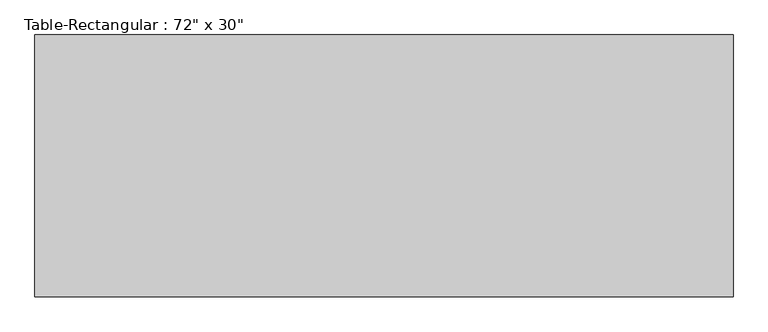
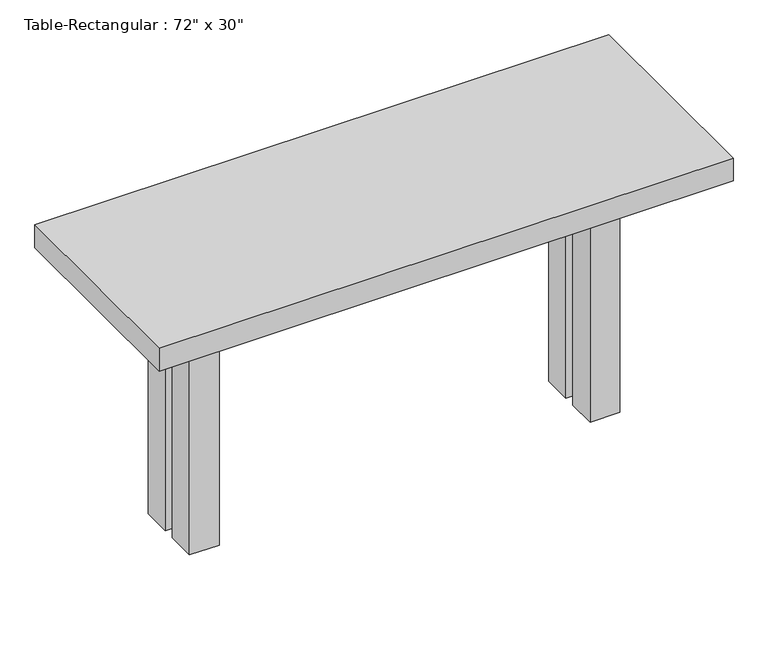
"""IFC4 building model written with IfcOpenShell, lengths in millimetres: furniture geometry."""

from ifc_helpers import new_model, si_unit, frame, origin, origin_with_axes, place, context, project, spatial, polyline, outline, extrude, source, transform, mapped, element, save


def furniture_c21ab0ed(model_context):
    return source(origin(), model_context, "Body", "SweptSolid", [
        extrude(outline(polyline([(393.7, 38.1), (393.7, 12.7), (-393.7, 12.7), (-393.7, 38.1), (393.7, 38.1)])), frame((0.0, 0.0, 457.2), z_axis=(0.0, 0.0, 1.0), x_axis=(1.0, 0.0, 0.0)), (0.0, 0.0, 1.0), 101.6),
        extrude(outline(polyline([(393.7, -38.1), (-393.7, -38.1), (-393.7, -12.7), (393.7, -12.7), (393.7, -38.1)])), frame((0.0, 0.0, 457.2), z_axis=(0.0, 0.0, 1.0), x_axis=(1.0, 0.0, 0.0)), (0.0, 0.0, 1.0), 101.6),
        extrude(outline(polyline([(-406.4, -12.7), (-431.8, -12.7), (-431.8, 12.7), (-406.4, 12.7), (-406.4, -12.7)])), frame((0.0, 0.0, 457.2), z_axis=(0.0, 0.0, 1.0), x_axis=(1.0, 0.0, 0.0)), (0.0, 0.0, 1.0), 101.6),
        extrude(outline(polyline([(406.4, -12.7), (406.4, 12.7), (431.8, 12.7), (431.8, -12.7), (406.4, -12.7)])), frame((0.0, 0.0, 457.2), z_axis=(0.0, 0.0, 1.0), x_axis=(1.0, 0.0, 0.0)), (0.0, 0.0, 1.0), 101.6),
        extrude(outline(polyline([(609.6, 228.6), (609.6, -228.6), (-609.6, -228.6), (-609.6, 228.6), (609.6, 228.6)])), frame((0.0, 0.0, 558.8), z_axis=(0.0, 0.0, 1.0), x_axis=(1.0, 0.0, 0.0)), (0.0, 0.0, 1.0), 50.8),
        extrude(outline(polyline([(-393.7, 76.2), (-393.7, 12.7), (-457.2, 12.7), (-457.2, 76.2), (-393.7, 76.2)])), origin_with_axes(), (0.0, 0.0, 1.0), 558.8),
        extrude(outline(polyline([(393.7, 76.2), (457.2, 76.2), (457.2, 12.7), (393.7, 12.7), (393.7, 76.2)])), origin_with_axes(), (0.0, 0.0, 1.0), 558.8),
        extrude(outline(polyline([(-393.7, -76.2), (-457.2, -76.2), (-457.2, -12.7), (-393.7, -12.7), (-393.7, -76.2)])), origin_with_axes(), (0.0, 0.0, 1.0), 558.8),
        extrude(outline(polyline([(393.7, -76.2), (393.7, -12.7), (457.2, -12.7), (457.2, -76.2), (393.7, -76.2)])), origin_with_axes(), (0.0, 0.0, 1.0), 558.8),
    ])


if __name__ == "__main__":
    model = new_model("IFC4")
    model_context = context("Model", 3, world=origin())
    ifc_project = project(units=[si_unit("LENGTHUNIT", "METRE", prefix="MILLI")], contexts=[model_context])
    site = spatial("IfcSite", under=ifc_project)
    building = spatial("IfcBuilding", under=site)
    placement = place(None, origin())
    furniture_shape = furniture_c21ab0ed(model_context)
    element("IfcFurniture", 1, ObjectType="Table-Rectangular : 72\" x 30\"", at=placement, inside=building, context=model_context, shape_type="MappedRepresentation", body=[
        mapped(furniture_shape, transform((0.0, 0.0, 0.0), x_axis=(1.0, 0.0, 0.0), y_axis=(0.0, 1.0, 0.0), z_axis=(0.0, 0.0, 1.0))),
    ])
    save(model, "model.ifc")

# Revit data of these elements
# Type "Table-Rectangular : 72\" x 30\""
#   Assembly Code = "E2020200"
#   Height = 2' - 0"
#   Length = 4' - 0"
#   Width = 1' - 6"
#   Base Material = Birch
#   Top Material = Birch
#   Default Elevation = 0
# Element 1 (IfcFurniture, "Table-Rectangular : 72\" x 30\"")
#   Materials on its faces: "Birch"
# Materials
#   "Birch": class "Wood", colour RGB 210 159 95, transparency 0, Description = "Betula Alleghaniensis", Cost = 0
